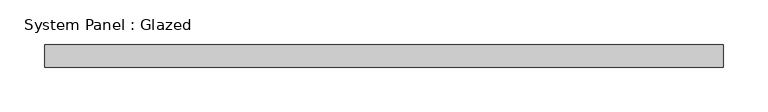
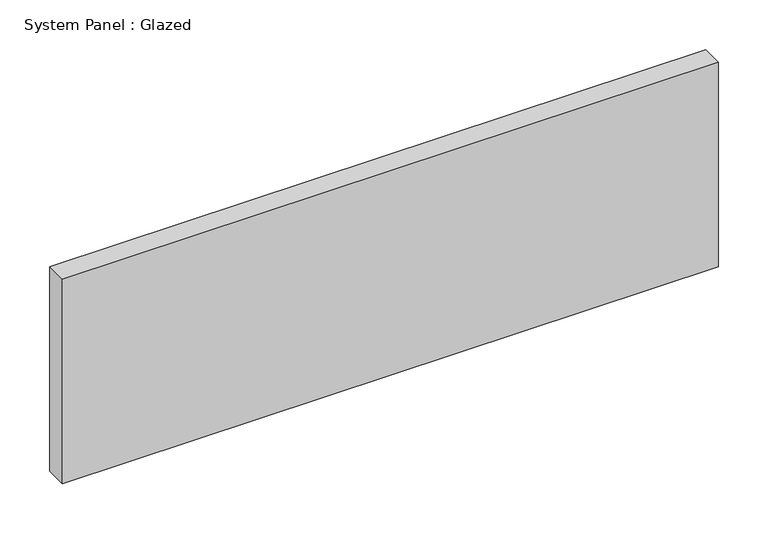
"""IFC4 building model written with IfcOpenShell, lengths in millimetres: plate geometry, System Panel : Glazed."""

from ifc_helpers import new_model, si_unit, origin, origin_with_axes, place, context, project, spatial, polyline, outline, extrude, source, transform, mapped, element, save


def system_panel_glazed_4c8acbbb(model_context):
    return source(origin(), model_context, "Body", "SweptSolid", [
        extrude(outline(polyline([(381.0, 19.05), (-381.0, 19.05), (-381.0, 44.45), (381.0, 44.45), (381.0, 19.05)])), origin_with_axes(), (0.0, 0.0, 1.0), 251.1186703),
    ])


if __name__ == "__main__":
    model = new_model("IFC4")
    model_context = context("Model", 3, world=origin())
    ifc_project = project(units=[si_unit("LENGTHUNIT", "METRE", prefix="MILLI")], contexts=[model_context])
    site = spatial("IfcSite", under=ifc_project)
    building = spatial("IfcBuilding", under=site)
    placement = place(None, origin())
    system_panel_glazed_shape = system_panel_glazed_4c8acbbb(model_context)
    element("IfcPlate", 1, ObjectType="System Panel : Glazed", at=placement, inside=building, context=model_context, shape_type="MappedRepresentation", body=[
        mapped(system_panel_glazed_shape, transform((0.0, 0.0, 0.0), x_axis=(1.0, 0.0, 0.0), y_axis=(0.0, 1.0, 0.0), z_axis=(0.0, 0.0, 1.0))),
    ])
    save(model, "model.ifc")

# Revit data of these elements
# Type "System Panel : Glazed"
#   Construction Type Id = "GSP4R"
#   Analytic Construction = "1/8 in Pilkington single glazing"
#   Visual Light Transmittance = 0.9
#   Solar Heat Gain Coefficient = 0.86
#   Heat Transfer Coefficient (U) = 1.18115 BTU/(h·ft²·°F)
#   Define Thermal Properties by = 1
# Element 1 (IfcPlate, "System Panel : Glazed")
#   Materials on its faces: "Glass"
# Materials
#   "Glass": class "Glass", colour RGB 0 128 192, transparency 0.75, Description = "Soda Lime Glass", Cost = 0
